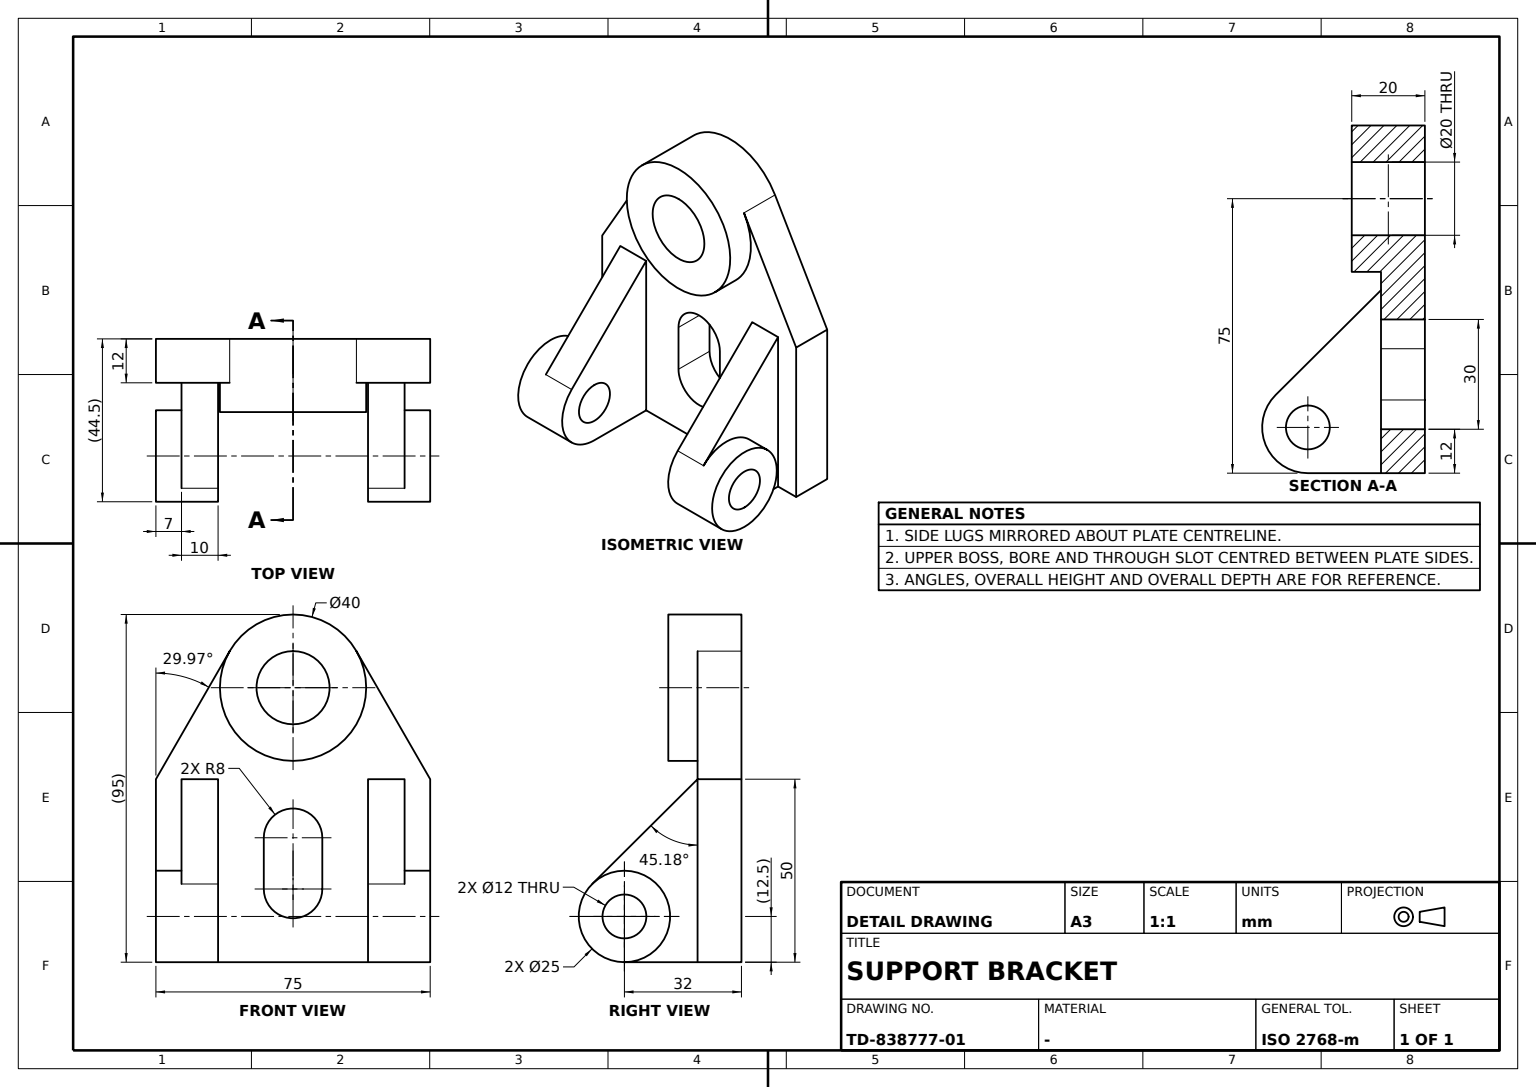
CATIA V5 part; units mm, degrees
sketch "Sketch1" plane through (0, 0, 0) normal (0, 1, 0) x (-1, 0, 0)
  circle A0 centre (0, 0) radius 20
  circle A1 centre (0, 0) radius 10
  dimension "radius A0" = 20
  dimension "radius A1" = 10
extrude "Pad1" add sketch "Sketch1" along normal mid plane 20
sketch "Sketch2" plane through (0, -10, 0) normal (0, -1, 0) x (1, 0, 0)
  point P0 (-17.3265, 9.9897)
  line L0 (-17.3265, 9.9897) -> (-37.5, -25)
  line L1 (-37.5, -25) -> (-37.5, -75)
  line L2 (-37.5, -75) -> (37.5, -75)
  line L3 (37.5, -75) -> (37.5, -25)
  line L4 (37.5, -25) -> (17.3265, 9.9897)
  point P1 (17.3265, 9.9897)
  circle A0 centre (0, 0) radius 20 construction
  circle A1 centre (0, 0) radius 20 construction
  circle A2 centre (0, 0) radius 20 construction
  circle A3 centre (0, 0) radius 20 construction
  arc A4 (-17.3265, 9.9897) -> (17.3265, 9.9897) centre (0, 0) ccw
  dimension "length L3" = 50
  dimension "length L1" = 50
  dimension "length L2" = 75
  dimension "distance L2 x axis" = 75
  constraint vertical L1 y-axis
  constraint vertical L3 y-axis
  constraint horizontal L2 x-axis
  constraint coincidence P0 A0
  constraint coincidence P1 A1
  constraint tangency L4 A2
  constraint tangency A3 L0
  constraint symmetry L1 L3 y-axis
extrude "Pad2" add sketch "Sketch2" against normal blind 12
sketch "Sketch3" plane through (37.5, 0, 0) normal (1, 0, 0) x (0, 1, 0)
  circle A0 centre (22, -62.5) radius 12.5
  point P0 (22, -62.5)
  line L0 (2, -75) -> (2, -25) construction
  line L1 (-10, -75) -> (2, -75) construction
  circle A1 centre (22, -62.5) radius 6
  dimension "radius A0" = 12.5
  dimension "distance L0 P0" = 20
  dimension "radius A1" = 6
  constraint tangency L1 A0
extrude "Pad3" add sketch "Sketch3" against normal blind 12
mirror "Mirror1" about plane through (0, 0, 0) normal (1, 0, 0) of "Pad3"
sketch "Sketch4" plane through (25.5, 0, 0) normal (-1, 0, 0) x (0, -1, 0)
  point P0 (-30.8115, -53.6339)
  line L0 (-30.8115, -53.6339) -> (-2, -25)
  line L1 (-2, -25) -> (-2, -75)
  line L2 (-2, -75) -> (-22, -75)
  point P1 (-22, -75)
  line L3 (-2, -25) -> (-2, -75) construction
  line L4 (10, -75) -> (-2, -75) construction
  circle A0 centre (-22, -62.5) radius 12.5 construction
  circle A1 centre (-22, -62.5) radius 12.5 construction
  circle A2 centre (-22, -62.5) radius 12.5 construction
  circle A3 centre (-22, -62.5) radius 12.5 construction
  arc A4 (-30.8115, -53.6339) -> (-22, -75) centre (-22, -62.5) ccw
  dimension "length L1" = 50
  constraint vertical L1 y-axis
  constraint horizontal L2 x-axis
  constraint coincidence L1 L3
  constraint coincidence L2 L4
  constraint coincidence P0 A0
  constraint coincidence P1 A1
  constraint tangency L2 A2
  constraint tangency L0 A3
  constraint tangency A4 L2
extrude "Pad4" add sketch "Sketch4" along normal mid plane 10
mirror "Mirror2" about plane through (0, 0, 0) normal (1, 0, 0) of "Pad4"
sketch "Pocket1 profile" plane through (30.5, 0, 0) normal (1, 0, 0) x (0, 1, 0)
  circle A0 centre (22, -62.5) radius 6
extrude "Pocket1" cut sketch "Pocket1 profile" against normal through all
sketch "Sketch5" plane through (0, 2, 0) normal (0, 1, 0) x (-1, 0, 0)
  arc A0 (8, -41) -> (-8, -41) centre (0, -41) ccw
  point P0 (0, -41)
  arc A1 (-8, -55) -> (8, -55) centre (0, -55) ccw
  point P1 (0, -55)
  point P2 (-8, -41)
  line L0 (-8, -41) -> (-8, -55)
  point P3 (-8, -55)
  point P4 (8, -55)
  point P5 (8, -41)
  line L1 (8, -41) -> (8, -55)
  point P6 (-8, -55)
  point P7 (8, -55)
  line L2 (-30.5, -75) -> (-37.5, -75) construction
  dimension "radius A1" = 8
  dimension "distance A1 A0" = 30
  dimension "distance P1 L2" = 20
  constraint coincidence P0 y-axis
  constraint coincidence P1 y-axis
  constraint coincidence L0 P6
  constraint coincidence L1 P7
  constraint coincidence P4 P7
  constraint vertical L0 y-axis
  constraint tangency L0 A0
  constraint tangency L0 A1
  constraint tangency A0 L1
  constraint symmetry P3 P4 y-axis
  constraint symmetry P2 P5 y-axis
  constraint symmetry L0 L1 y-axis
extrude "Pocket2" cut sketch "Sketch5" against normal through all
